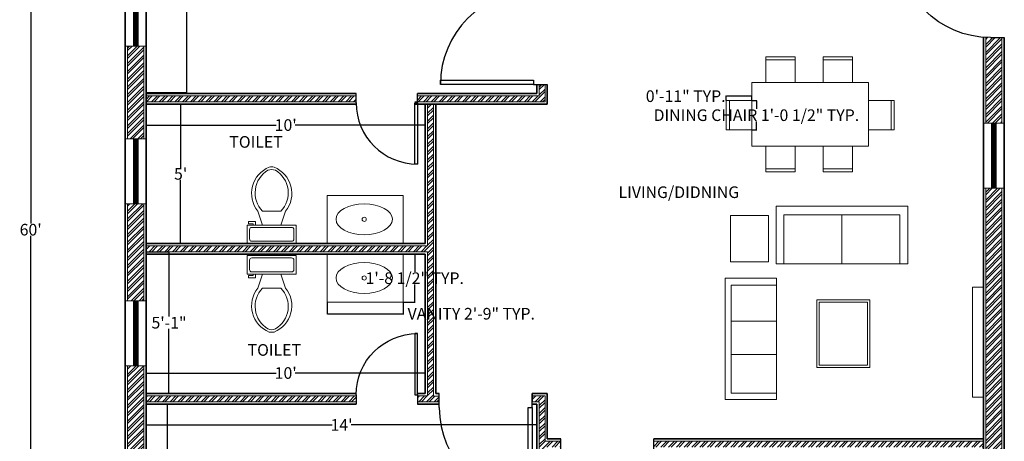
# Model space of a CAD drawing. Units: inches. Extents: x 210 to 633, y 286 to 1043.
# Tile 2 of 3: x 210 to 633, y 555 to 736. Entities that reach past the tile are written whole.
import ezdxf

# ---------------------------------------------------------------- set-up
doc = ezdxf.new("R2010")
doc.units = ezdxf.units.IN
doc.header["$MEASUREMENT"] = 0
for name, color, linetype, lineweight in [('A-ANNO-DIMS', 170, 'Continuous', 18), ('A-AREA-IDEN', 7, 'Continuous', 25), ('A-DOOR', 4, 'Continuous', 25), ('A-FLOR-FIXT', 210, 'Continuous', 18), ('A-GLAZ-PATT', 130, 'Continuous', 13), ('A-WALL-PATT', 35, 'Continuous', 13), ('fur', 210, 'Continuous', 18), ('wall', 10, 'Continuous', 35), ('wind', 130, 'Continuous', 18)]:
    doc.layers.add(name, color=color, linetype=linetype, lineweight=lineweight)
doc.styles.get("Standard").update_dxf_attribs({"font": 'arial.ttf'})
doc.dimstyles.get("Standard").update_dxf_attribs({"dimtxt": 5, "dimasz": 0.18, "dimexe": 0.18, "dimexo": 0.0625, "dimgap": 0.09, "dimtad": 0, "dimtih": 1, "dimtoh": 1, "dimdec": 0, "dimzin": 0, "dimdsep": 46, "dimlunit": 4, "dimtxsty": 'Standard', "dimcen": 0.09, "dimadec": 0, "dimazin": 0, "dimtfac": 1, "dimtdec": 0, "dimtofl": 0, "dimtmove": 0, "dimatfit": 3, "dimfxl": 1, "dimtolj": 1, "dimtzin": 0, "dimarcsym": 0})

# ---------------------------------------------------------------- blocks, each defined once
blk = doc.blocks.new('*U2')
for p, q in [((0, 0), (0, -6)), ((40, 0), (40, -6))]:
    blk.add_line(p, q)
blk.add_lwpolyline([(0, 0), (0, 40), (1.75, 40), (1.75, 0)], close=True)
blk.add_arc((0, 0), 40, 0, 90)
blk = doc.blocks.new('*U4')
for p, q in [((9.5, -6), (9.5, -2)), ((-8, -8.5), (-8, -8)), ((-7, -8), (-7, -9.5)), ((-4, -8), (-6, -14)), ((4, -8), (6, -14)), ((-10, -8.5), (-8, -8.5)), ((-10, -9.5), (-10, -8.5)), ((-7, -9.5), (-10, -9.5)), ((4, -14), (-4, -14))]:
    blk.add_line(p, q)
blk.add_lwpolyline([(10.5, -8), (10.5, 0), (-10.5, 0), (-10.5, -8)], close=True)
for points in [[(-9.5, -2), (-9.5, -6)], [(8.5, -1), (-8.5, -1)], [(-8.5, -7), (8.5, -7)]]:
    blk.add_lwpolyline(points)
for centre, radius, start, end in [((-8.62, -1.88), 0.884, 81.8699, 188.1301), ((8.62, -1.88), 0.884, 351.8699, 98.1301), ((-8.62, -6.12), 0.884, 171.8699, 278.1301), ((8.62, -6.12), 0.884, 261.8699, 8.1301), ((3.52, -21.58), 12.17, 141.4691, 247.9714), ((4.2, -21.82), 11.33, 136.3677, 238.9468), ((-3.52, -21.58), 12.17, 292.0284, 38.5307), ((-4.2, -21.82), 11.33, 301.053, 43.6321), ((0, -27.88), 4, 245.7318, 294.2682), ((0, -29), 4, 254.8605, 285.1395)]:
    blk.add_arc(centre, radius, start, end)
blk = doc.blocks.new('*D20')
at = {"layer": 'A-ANNO-DIMS', "color": 0, "lineweight": -2, "transparency": 16777216}
for p, q in [((264.44, 848.52), (282.01, 848.52)), ((281.83, 848.34), (281.83, 779.38)), ((281.83, 705.21), (281.83, 774.18)), ((264.44, 705.03), (282.01, 705.03))]:
    blk.add_line(p, q, dxfattribs=at)
at = {"layer": 'A-ANNO-DIMS', "color": 0, "transparency": 16777216}
for points in [[(281.8, 848.34), (281.86, 848.34), (281.83, 848.52)], [(281.8, 705.21), (281.86, 705.21), (281.83, 705.03)]]:
    blk.add_solid(points, dxfattribs=at)
at = {"layer": 'Defpoints', "color": 0, "transparency": 16777216}
for p in [(264.37, 848.52), (281.83, 848.52), (264.37, 705.03)]:
    blk.add_point(p, dxfattribs=at)
at = {"layer": 'A-ANNO-DIMS', "color": 0, "transparency": 16777216, "insert": (281.83, 776.78), "char_height": 5, "attachment_point": 5}
blk.add_mtext('\\A1;11\'-11"', dxfattribs=at)
blk = doc.blocks.new('*D21')
at = {"layer": 'A-ANNO-DIMS', "color": 0, "lineweight": -2, "transparency": 16777216}
for p, q in [((264.37, 699.96), (264.37, 690.83)), ((384.37, 699.96), (384.37, 690.83)), ((264.55, 691.01), (320.28, 691.01)), ((384.19, 691.01), (328.47, 691.01))]:
    blk.add_line(p, q, dxfattribs=at)
at = {"layer": 'A-ANNO-DIMS', "color": 0, "transparency": 16777216}
for points in [[(264.55, 691.04), (264.55, 690.98), (264.37, 691.01)], [(384.19, 691.04), (384.19, 690.98), (384.37, 691.01)]]:
    blk.add_solid(points, dxfattribs=at)
at = {"layer": 'Defpoints', "color": 0, "transparency": 16777216}
for p in [(264.37, 700.02), (384.37, 700.02), (384.37, 691.01)]:
    blk.add_point(p, dxfattribs=at)
at = {"layer": 'A-ANNO-DIMS', "color": 0, "transparency": 16777216, "insert": (324.37, 691.01), "char_height": 5, "attachment_point": 5}
blk.add_mtext("\\A1;10'", dxfattribs=at)
blk = doc.blocks.new('*D22')
at = {"layer": 'A-ANNO-DIMS', "color": 0, "lineweight": -2, "transparency": 16777216}
for p, q in [((264.44, 700.02), (279.37, 700.02)), ((279.19, 699.84), (279.19, 672.65)), ((279.19, 640.2), (279.19, 667.39)), ((264.44, 640.02), (279.37, 640.02))]:
    blk.add_line(p, q, dxfattribs=at)
at = {"layer": 'A-ANNO-DIMS', "color": 0, "transparency": 16777216}
for points in [[(279.16, 699.84), (279.22, 699.84), (279.19, 700.02)], [(279.16, 640.2), (279.22, 640.2), (279.19, 640.02)]]:
    blk.add_solid(points, dxfattribs=at)
at = {"layer": 'Defpoints', "color": 0, "transparency": 16777216}
for p in [(264.37, 700.02), (279.19, 700.02), (264.37, 640.02)]:
    blk.add_point(p, dxfattribs=at)
at = {"layer": 'A-ANNO-DIMS', "color": 0, "transparency": 16777216, "insert": (279.19, 670.02), "char_height": 5, "attachment_point": 5}
blk.add_mtext("\\A1;5'", dxfattribs=at)
blk = doc.blocks.new('*D23')
at = {"layer": 'A-ANNO-DIMS', "color": 0, "lineweight": -2, "transparency": 16777216}
for p, q in [((264.44, 636.52), (274.36, 636.52)), ((274.18, 636.34), (274.18, 608.66)), ((274.18, 575.7), (274.18, 603.38)), ((264.44, 575.52), (274.36, 575.52))]:
    blk.add_line(p, q, dxfattribs=at)
at = {"layer": 'A-ANNO-DIMS', "color": 0, "transparency": 16777216}
for points in [[(274.15, 636.34), (274.21, 636.34), (274.18, 636.52)], [(274.15, 575.7), (274.21, 575.7), (274.18, 575.52)]]:
    blk.add_solid(points, dxfattribs=at)
at = {"layer": 'Defpoints', "color": 0, "transparency": 16777216}
for p in [(264.37, 636.52), (274.18, 636.52), (264.37, 575.52)]:
    blk.add_point(p, dxfattribs=at)
at = {"layer": 'A-ANNO-DIMS', "color": 0, "transparency": 16777216, "insert": (274.18, 606.02), "char_height": 5, "attachment_point": 5}
blk.add_mtext('\\A1;5\'-1"', dxfattribs=at)
blk = doc.blocks.new('*D24')
at = {"layer": 'A-ANNO-DIMS', "color": 0, "lineweight": -2, "transparency": 16777216}
for p, q in [((264.37, 635.46), (264.37, 584.21)), ((384.37, 635.46), (384.37, 584.21)), ((264.55, 584.39), (320.28, 584.39)), ((384.19, 584.39), (328.47, 584.39))]:
    blk.add_line(p, q, dxfattribs=at)
at = {"layer": 'A-ANNO-DIMS', "color": 0, "transparency": 16777216}
for points in [[(264.55, 584.42), (264.55, 584.36), (264.37, 584.39)], [(384.19, 584.42), (384.19, 584.36), (384.37, 584.39)]]:
    blk.add_solid(points, dxfattribs=at)
at = {"layer": 'Defpoints', "color": 0, "transparency": 16777216}
for p in [(264.37, 635.52), (384.37, 635.52), (384.37, 584.39)]:
    blk.add_point(p, dxfattribs=at)
at = {"layer": 'A-ANNO-DIMS', "color": 0, "transparency": 16777216, "insert": (324.37, 584.39), "char_height": 5, "attachment_point": 5}
blk.add_mtext("\\A1;10'", dxfattribs=at)
blk = doc.blocks.new('*D25')
at = {"layer": 'A-ANNO-DIMS', "color": 0, "lineweight": -2, "transparency": 16777216}
for p, q in [((264.37, 570.96), (264.37, 561.9)), ((432.37, 570.96), (432.37, 561.9)), ((264.55, 562.08), (344.28, 562.08)), ((432.19, 562.08), (352.47, 562.08))]:
    blk.add_line(p, q, dxfattribs=at)
at = {"layer": 'A-ANNO-DIMS', "color": 0, "transparency": 16777216}
for points in [[(264.55, 562.11), (264.55, 562.05), (264.37, 562.08)], [(432.19, 562.11), (432.19, 562.05), (432.37, 562.08)]]:
    blk.add_solid(points, dxfattribs=at)
at = {"layer": 'Defpoints', "color": 0, "transparency": 16777216}
for p in [(264.37, 571.02), (432.37, 571.02), (432.37, 562.08)]:
    blk.add_point(p, dxfattribs=at)
at = {"layer": 'A-ANNO-DIMS', "color": 0, "transparency": 16777216, "insert": (348.37, 562.08), "char_height": 5, "attachment_point": 5}
blk.add_mtext("\\A1;14'", dxfattribs=at)
blk = doc.blocks.new('*D26')
at = {"layer": 'A-ANNO-DIMS', "color": 0, "lineweight": -2, "transparency": 16777216}
for p, q in [((264.44, 571.02), (273.63, 571.02)), ((273.45, 570.84), (273.45, 501.62)), ((273.45, 427.2), (273.45, 496.42)), ((264.44, 427.02), (273.63, 427.02))]:
    blk.add_line(p, q, dxfattribs=at)
at = {"layer": 'A-ANNO-DIMS', "color": 0, "transparency": 16777216}
for points in [[(273.42, 570.84), (273.48, 570.84), (273.45, 571.02)], [(273.42, 427.2), (273.48, 427.2), (273.45, 427.02)]]:
    blk.add_solid(points, dxfattribs=at)
at = {"layer": 'Defpoints', "color": 0, "transparency": 16777216}
for p in [(264.37, 571.02), (264.37, 427.02), (273.45, 427.02)]:
    blk.add_point(p, dxfattribs=at)
at = {"layer": 'A-ANNO-DIMS', "color": 0, "transparency": 16777216, "insert": (273.45, 499.02), "char_height": 5, "attachment_point": 5}
blk.add_mtext("\\A1;12'", dxfattribs=at)
blk = doc.blocks.new('*D36')
at = {"layer": 'A-ANNO-DIMS', "color": 0, "lineweight": -2, "transparency": 16777216}
for p, q in [((255.31, 1006.02), (214.53, 1006.02)), ((214.71, 1005.84), (214.71, 648.66)), ((214.71, 286.2), (214.71, 643.38)), ((255.31, 286.02), (214.53, 286.02))]:
    blk.add_line(p, q, dxfattribs=at)
at = {"layer": 'A-ANNO-DIMS', "color": 0, "transparency": 16777216}
for points in [[(214.68, 1005.84), (214.74, 1005.84), (214.71, 1006.02)], [(214.68, 286.2), (214.74, 286.2), (214.71, 286.02)]]:
    blk.add_solid(points, dxfattribs=at)
at = {"layer": 'Defpoints', "color": 0, "transparency": 16777216}
for p in [(214.71, 1006.02), (255.37, 1006.02), (255.37, 286.02)]:
    blk.add_point(p, dxfattribs=at)
at = {"layer": 'A-ANNO-DIMS', "color": 0, "transparency": 16777216, "insert": (214.71, 646.02), "char_height": 5, "attachment_point": 5}
blk.add_mtext("\\A1;60'", dxfattribs=at)
blk = doc.blocks.new('CHAIR-DINING')
blk.add_line((0, 9.71), (12.58, 9.71))
blk.add_lwpolyline([(0, 0), (12.58, 0), (12.58, 11.05), (0, 11.05)], close=True)
blk = doc.blocks.new('BASIN-VANITY')
blk.add_lwpolyline([(0, 0), (32.77, 0), (32.77, 20.73), (0, 20.73)], close=True)
blk.add_circle((15.97, 10.46), 0.893)
blk.add_ellipse((15.97, 10.46), major_axis=(12.12, 0), ratio=0.5487)
blk = doc.blocks.new('*D43')
at = {"layer": 'A-ANNO-DIMS', "color": 0, "lineweight": -2, "transparency": 16777216}
for p, q in [((524.94, 701.54), (526.94, 701.54)), ((526.76, 701.36), (526.76, 697.93)), ((526.76, 689.14), (526.76, 692.58)), ((524.94, 688.96), (526.94, 688.96))]:
    blk.add_line(p, q, dxfattribs=at)
at = {"layer": 'A-ANNO-DIMS', "color": 0, "transparency": 16777216}
for points in [[(526.73, 701.36), (526.79, 701.36), (526.76, 701.54)], [(526.73, 689.14), (526.79, 689.14), (526.76, 688.96)]]:
    blk.add_solid(points, dxfattribs=at)
at = {"layer": 'Defpoints', "color": 0, "transparency": 16777216}
for p in [(524.87, 701.54), (526.76, 701.54), (524.87, 688.96)]:
    blk.add_point(p, dxfattribs=at)
at = {"layer": 'A-ANNO-DIMS', "color": 0, "transparency": 16777216, "insert": (526.76, 695.25), "char_height": 5, "attachment_point": 5}
blk.add_mtext('\\A1;DINING CHAIR 1\'-0 1/2" TYP.', dxfattribs=at)
blk = doc.blocks.new('*D44')
at = {"layer": 'A-ANNO-DIMS', "color": 0, "lineweight": -2, "transparency": 16777216}
for p, q in [((513.82, 703.43), (513.64, 703.43)), ((513.82, 701.6), (513.82, 703.61)), ((524.69, 703.43), (514, 703.43)), ((524.87, 701.6), (524.87, 703.61))]:
    blk.add_line(p, q, dxfattribs=at)
at = {"layer": 'A-ANNO-DIMS', "color": 0, "transparency": 16777216}
for points in [[(514, 703.46), (514, 703.4), (513.82, 703.43)], [(524.69, 703.46), (524.69, 703.4), (524.87, 703.43)]]:
    blk.add_solid(points, dxfattribs=at)
at = {"layer": 'Defpoints', "color": 0, "transparency": 16777216}
for p in [(513.82, 703.43), (513.82, 701.54), (524.87, 701.54)]:
    blk.add_point(p, dxfattribs=at)
at = {"layer": 'A-ANNO-DIMS', "color": 0, "transparency": 16777216, "insert": (496.37, 703.43), "char_height": 5, "attachment_point": 5}
blk.add_mtext('\\A1;0\'-11" TYP.', dxfattribs=at)
blk = doc.blocks.new('*D45')
at = {"layer": 'A-ANNO-DIMS', "color": 0, "lineweight": -2, "transparency": 16777216}
for p, q in [((342.16, 614.73), (342.16, 609.7)), ((374.94, 614.73), (374.94, 609.7)), ((342.34, 609.88), (374.76, 609.88)), ((374.94, 609.88), (375.12, 609.88))]:
    blk.add_line(p, q, dxfattribs=at)
at = {"layer": 'A-ANNO-DIMS', "color": 0, "transparency": 16777216}
for points in [[(342.34, 609.91), (342.34, 609.85), (342.16, 609.88)], [(374.76, 609.91), (374.76, 609.85), (374.94, 609.88)]]:
    blk.add_solid(points, dxfattribs=at)
at = {"layer": 'Defpoints', "color": 0, "transparency": 16777216}
for p in [(342.16, 614.79), (374.94, 614.79), (374.94, 609.88)]:
    blk.add_point(p, dxfattribs=at)
at = {"layer": 'A-ANNO-DIMS', "color": 0, "transparency": 16777216, "insert": (404.16, 609.88), "char_height": 5, "attachment_point": 5}
blk.add_mtext('\\A1;VANITY 2\'-9" TYP.', dxfattribs=at)
blk = doc.blocks.new('*D46')
at = {"layer": 'A-ANNO-DIMS', "color": 0, "lineweight": -2, "transparency": 16777216}
for p, q in [((375, 635.52), (380.03, 635.52)), ((379.85, 635.34), (379.85, 627.83)), ((379.85, 614.97), (379.85, 622.48)), ((375, 614.79), (380.03, 614.79))]:
    blk.add_line(p, q, dxfattribs=at)
at = {"layer": 'A-ANNO-DIMS', "color": 0, "transparency": 16777216}
for points in [[(379.82, 635.34), (379.88, 635.34), (379.85, 635.52)], [(379.82, 614.97), (379.88, 614.97), (379.85, 614.79)]]:
    blk.add_solid(points, dxfattribs=at)
at = {"layer": 'Defpoints', "color": 0, "transparency": 16777216}
for p in [(374.94, 635.52), (379.85, 635.52), (374.94, 614.79)]:
    blk.add_point(p, dxfattribs=at)
at = {"layer": 'A-ANNO-DIMS', "color": 0, "transparency": 16777216, "insert": (379.85, 625.16), "char_height": 5, "attachment_point": 5}
blk.add_mtext('\\A1;1\'-8 1/2" TYP.', dxfattribs=at)

msp = doc.modelspace()

# ---------------------------------------------------------------- hatches: boundary and pattern name
at = {"layer": 'A-GLAZ-PATT'}
h = msp.add_hatch(dxfattribs=at)
h.set_pattern_fill('ANSI31', color=256)
h.paths.add_polyline_path([(580.59, 368.5), (495.79, 368.5), (495.79, 366.5), (580.59, 366.5)])
h.paths.add_polyline_path([(629.87, 441.57), (627.87, 441.57), (627.87, 386.08), (629.87, 386.08)])
h.paths.add_polyline_path([(260.87, 537.72), (258.87, 537.72), (258.87, 447.09), (260.87, 447.09)])
h.paths.add_polyline_path([(260.87, 615.48), (258.87, 615.48), (258.87, 587.48), (260.87, 587.48)])
h.paths.add_polyline_path([(260.87, 685.1), (258.87, 685.1), (258.87, 657.11), (260.87, 657.11)])
h.paths.add_polyline_path([(629.87, 691.84), (627.87, 691.84), (627.87, 663.85), (629.87, 663.85)])
h.paths.add_polyline_path([(260.87, 815.6), (258.87, 815.6), (258.87, 724.96), (260.87, 724.96)])
h.paths.add_polyline_path([(629.87, 831.37), (627.87, 831.37), (627.87, 803.38), (629.87, 803.38)])
h.paths.add_polyline_path([(629.87, 963.44), (627.87, 963.44), (627.87, 872.81), (629.87, 872.81)])
h.paths.add_polyline_path([(495.13, 1002.52), (448.67, 1002.52), (448.67, 1000.52), (495.13, 1000.52)])
h.paths.add_polyline_path([(417.29, 1002.52), (370.83, 1002.52), (370.83, 1000.52), (417.29, 1000.52)])
h.paths.add_polyline_path([(260.87, 971.49), (258.87, 971.49), (258.87, 880.85), (260.87, 880.85)])
at = {"layer": 'A-WALL-PATT'}
h = msp.add_hatch(dxfattribs=at)
h.set_pattern_fill('ANSI32', color=256, scale=6.3)
h.paths.add_polyline_path([(370.83, 1005.02), (256.37, 1005.02), (256.37, 971.49), (263.37, 971.49), (263.37, 998.02), (370.83, 998.02)])
h.paths.add_polyline_path([(448.67, 1005.02), (417.29, 1005.02), (417.29, 998.02), (432.37, 998.02), (448.67, 998.02)])
h.paths.add_polyline_path([(632.37, 1005.02), (495.13, 1005.02), (495.13, 998.02), (508.87, 998.02), (625.37, 998.02), (625.37, 963.44), (632.37, 963.44)])
h.paths.add_polyline_path([(263.37, 849.52), (433.37, 849.52), (433.37, 748.51), (435.87, 748.51), (435.87, 849.52), (435.87, 858.43), (433.37, 858.43), (433.37, 852.02), (263.37, 852.02), (263.37, 880.85), (256.37, 880.85), (256.37, 815.6), (263.37, 815.6)])
h.paths.add_polyline_path([(263.37, 724.96), (256.37, 724.96), (256.37, 685.1), (263.37, 685.1)])
h.paths.add_polyline_path([(354.65, 703.52), (264.37, 703.52), (264.37, 701.02), (354.65, 701.02)])
h.paths.add_polyline_path([(263.37, 657.11), (256.37, 657.11), (256.37, 615.48), (263.37, 615.48)])
h = msp.add_hatch(dxfattribs=at)
h.set_pattern_fill('ANSI32', color=256, scale=6.3)
h.paths.add_polyline_path([(551.37, 786.25), (548.87, 786.25), (548.87, 773.02), (625.37, 773.02), (625.37, 768.63), (627.37, 768.63), (632.37, 768.63), (632.37, 803.38), (625.37, 803.38), (625.37, 775.52), (551.37, 775.52)])
h.paths.add_polyline_path([(435.87, 997.02), (433.37, 997.02), (433.37, 898.43), (435.87, 898.43), (435.87, 909.52), (440.28, 909.52), (440.28, 912.02), (435.87, 912.02)])
h.paths.add_polyline_path([(512.37, 997.02), (509.87, 997.02), (509.87, 912.02), (466.62, 912.02), (466.62, 909.52), (512.37, 909.52)])
h.paths.add_polyline_path([(435.87, 708.51), (433.37, 708.51), (433.37, 703.52), (381, 703.52), (381, 701.02), (435.87, 701.02)])
h.paths.add_polyline_path([(387.87, 700.02), (385.37, 700.02), (385.37, 639.02), (264.37, 639.02), (264.37, 636.52), (385.37, 636.52), (385.37, 574.52), (381, 574.52), (381, 572.02), (390.4, 572.02), (390.4, 574.43), (387.87, 574.43), (387.87, 635.52)])
h = msp.add_hatch(dxfattribs=at)
h.set_pattern_fill('ANSI32', color=256, scale=6.3)
h.paths.add_polyline_path([(502.57, 551.52), (500.07, 551.52), (500.07, 537.88), (502.57, 537.88)])
h.paths.add_polyline_path([(632.37, 728.63), (627.37, 728.63, -0.012506), (625.37, 728.68), (625.37, 691.84), (632.37, 691.84)])
h = msp.add_hatch(dxfattribs=at)
h.set_pattern_fill('ANSI32', color=256, scale=6.3)
h.paths.add_polyline_path([(632.37, 663.85), (625.37, 663.85), (625.37, 556.02), (625.37, 441.57), (632.37, 441.57)])
h.paths.add_polyline_path([(632.37, 386.08), (625.37, 386.08), (625.37, 289.52), (625.37, 286.02), (632.37, 286.02), (632.37, 287.02)])
h.paths.add_polyline_path([(624.37, 371), (580.59, 371), (580.59, 364), (624.37, 364)])
h.paths.add_polyline_path([(495.79, 371), (436.87, 371), (436.87, 364), (495.79, 364)])
h = msp.add_hatch(dxfattribs=at)
h.set_pattern_fill('ANSI32', color=256, scale=6.3)
h.paths.add_polyline_path([(263.37, 587.48), (256.37, 587.48), (256.37, 537.72), (263.37, 537.72)])
h.paths.add_polyline_path([(354.65, 574.52), (264.37, 574.52), (264.37, 572.02), (354.65, 572.02)])
h = msp.add_hatch(dxfattribs=at)
h.set_pattern_fill('ANSI32', color=256, scale=6.3)
h.paths.add_polyline_path([(442.64, 555.02), (435.87, 555.02), (435.87, 552.52), (442.64, 552.52)])
h.paths.add_polyline_path([(435.87, 574.52), (433.37, 574.52), (433.37, 414.65), (435.87, 414.65)])
h.paths.add_polyline_path([(433.37, 574.52), (430.4, 574.52), (430.4, 572.02), (433.37, 572.02)])
h = msp.add_hatch(dxfattribs=at)
h.set_pattern_fill('ANSI32', color=256, scale=6.3)
h.paths.add_polyline_path([(624.37, 555.02), (482.64, 555.02), (482.64, 552.52), (624.37, 552.52)])

# ---------------------------------------------------------------- linework, layer by layer
for p, q in [((625.37, 728.74), (625.37, 691.84)), ((632.37, 691.84), (632.37, 728.63)), ((256.37, 724.96), (256.37, 685.1)), ((263.37, 724.96), (263.37, 685.1)), ((433.37, 703.52), (433.37, 708.51)), ((435.87, 701.02), (435.87, 708.51)), ((264.37, 703.52), (354.65, 703.52)), ((381, 703.52), (433.37, 703.52)), ((264.37, 701.02), (354.66, 701.02)), ((379.84, 701.02), (435.87, 701.02)), ((385.37, 639.02), (385.37, 700.02)), ((387.87, 635.52), (387.87, 700.02)), ((625.37, 663.85), (625.37, 556.02)), ((632.37, 441.57), (632.37, 663.85)), ((256.37, 657.11), (256.37, 615.48)), ((263.37, 657.11), (263.37, 615.48)), ((264.37, 639.02), (385.37, 639.02)), ((264.37, 636.52), (385.37, 636.52)), ((385.37, 574.52), (385.37, 636.52)), ((387.87, 574.43), (387.87, 635.52)), ((256.37, 587.48), (256.37, 537.72)), ((263.37, 587.48), (263.37, 537.72)), ((264.37, 574.52), (354.66, 574.52)), ((264.37, 572.02), (354.65, 572.02)), ((381, 574.52), (385.37, 574.52)), ((381, 572.02), (390.4, 572.02)), ((387.87, 574.43), (390.4, 574.43)), ((435.87, 574.52), (430.4, 574.52)), ((430.4, 572.02), (430.4, 574.52)), ((430.4, 574.52), (435.87, 574.52)), ((433.37, 572.02), (430.4, 572.02)), ((433.37, 572.02), (430.4, 572.02)), ((433.37, 426.02), (433.37, 572.02)), ((433.37, 426.02), (433.37, 572.02)), ((435.87, 555.02), (435.87, 574.52)), ((435.87, 574.52), (435.87, 555.02)), ((442.64, 555.02), (435.87, 555.02)), ((435.87, 555.02), (442.64, 555.02)), ((442.64, 555.02), (442.64, 552.52)), ((624.37, 555.02), (482.64, 555.02)), ((625.37, 556.02), (625.37, 441.57))]:
    msp.add_line(p, q, dxfattribs=at)
at = {"layer": 'fur'}
for p, q in [((538.5, 631.27), (538.5, 652.34)), ((538.5, 652.34), (588.43, 652.34)), ((563.47, 652.34), (563.57, 631.27)), ((588.43, 652.34), (588.43, 631.27)), ((515.96, 575.75), (515.96, 622.22)), ((515.96, 622.22), (535.48, 622.22)), ((535.48, 606.69), (515.96, 606.69)), ((535.48, 592.34), (515.96, 592.34)), ((535.48, 575.75), (515.96, 575.75))]:
    msp.add_line(p, q, dxfattribs=at)
for points in [[(575, 709.36), (524.87, 709.36), (524.87, 681.95), (575, 681.95)], [(531.93, 632.23), (515.59, 632.23), (515.59, 652.09), (531.93, 652.09)], [(535.2, 656.2), (591.94, 656.2), (591.94, 631.27), (535.2, 631.27)], [(535.48, 625.11), (513.41, 625.11), (513.41, 572.96), (535.48, 572.96)], [(624.37, 621.27), (619.7, 621.27), (619.7, 573.99), (624.37, 573.99)], [(552.78, 615.9), (575.55, 615.9), (575.55, 586.72), (552.78, 586.72)], [(553.78, 614.9), (574.55, 614.9), (574.55, 587.72), (553.78, 587.72)]]:
    msp.add_lwpolyline(points, close=True, dxfattribs=at)
at = {"layer": 'wall'}
for p, q in [((255.37, 1006.02), (255.37, 286.02)), ((264.37, 848.52), (264.37, 704.52)), ((264.37, 848.52), (264.37, 427.02)), ((624.37, 290.52), (624.37, 728.74)), ((624.37, 728.74), (624.37, 556.02)), ((624.37, 728.74), (624.37, 691.84)), ((633.37, 286.02), (633.37, 728.63)), ((633.37, 691.84), (633.37, 728.63)), ((255.37, 685.1), (255.37, 724.96)), ((264.37, 685.1), (264.37, 724.96)), ((432.37, 704.52), (432.37, 708.51)), ((432.37, 704.52), (432.37, 708.51)), ((436.87, 700.02), (436.87, 708.51)), ((436.87, 700.02), (436.87, 708.51)), ((264.37, 704.52), (354.65, 704.52)), ((264.37, 704.52), (354.65, 704.52)), ((381, 704.52), (432.37, 704.52)), ((381, 704.52), (432.37, 704.52)), ((264.37, 700.02), (354.66, 700.02)), ((264.37, 700.02), (264.37, 640.02)), ((264.37, 700.02), (354.66, 700.02)), ((379.84, 700.02), (436.87, 700.02)), ((381, 700.02), (436.87, 700.02)), ((384.37, 640.02), (384.37, 700.02)), ((384.37, 640.02), (384.37, 700.02)), ((388.87, 635.52), (388.87, 700.02)), ((388.87, 575.52), (388.87, 700.02)), ((624.37, 663.85), (624.37, 441.57)), ((633.37, 441.57), (633.37, 663.85)), ((255.37, 615.48), (255.37, 657.11)), ((264.37, 615.48), (264.37, 657.11)), ((264.37, 640.02), (384.37, 640.02)), ((264.37, 640.02), (384.37, 640.02)), ((264.37, 635.52), (384.37, 635.52)), ((264.37, 635.52), (264.37, 575.52)), ((384.37, 635.52), (264.37, 635.52)), ((384.37, 575.52), (384.37, 635.52)), ((384.37, 575.52), (384.37, 635.52)), ((388.87, 575.52), (388.87, 635.52)), ((255.37, 537.72), (255.37, 587.48)), ((264.37, 587.48), (264.37, 537.72)), ((264.37, 575.52), (354.66, 575.52)), ((354.66, 575.52), (264.37, 575.52)), ((381, 575.52), (384.37, 575.52)), ((381, 575.52), (384.37, 575.52)), ((390.4, 575.52), (388.87, 575.52)), ((390.4, 575.52), (388.87, 575.52)), ((436.87, 575.52), (430.4, 575.52)), ((436.87, 575.52), (430.4, 575.52)), ((430.4, 572.02), (430.4, 575.52)), ((436.87, 556.02), (436.87, 575.52)), ((436.87, 556.02), (436.87, 575.52)), ((264.37, 571.02), (354.65, 571.02)), ((264.37, 571.02), (264.37, 427.02)), ((264.37, 571.02), (354.65, 571.02)), ((381, 571.02), (390.4, 571.02)), ((381, 571.02), (390.4, 571.02)), ((390.4, 571.02), (388.87, 571.02)), ((432.37, 571.02), (430.4, 571.02)), ((430.4, 571.02), (432.37, 571.02)), ((432.37, 427.02), (432.37, 571.02)), ((432.37, 571.02), (432.37, 427.02)), ((442.64, 556.02), (436.87, 556.02)), ((442.64, 556.02), (436.87, 556.02)), ((624.37, 556.02), (482.64, 556.02)), ((624.37, 556.02), (482.64, 556.02))]:
    msp.add_line(p, q, dxfattribs=at)
at = {"layer": 'wind'}
for p, q in [((258.87, 724.96), (258.87, 815.6)), ((258.87, 724.96), (258.87, 815.6)), ((260.87, 724.96), (260.87, 815.6)), ((627.87, 663.85), (627.87, 691.84)), ((629.87, 663.85), (629.87, 691.84)), ((258.87, 657.11), (258.87, 685.1)), ((260.87, 657.11), (260.87, 685.1)), ((258.87, 587.48), (258.87, 615.48)), ((260.87, 587.48), (260.87, 615.48))]:
    msp.add_line(p, q, dxfattribs=at)
for points in [[(264.37, 724.96), (255.37, 724.96), (255.37, 815.6), (264.37, 815.6)], [(633.37, 691.84), (624.37, 691.84), (624.37, 663.85), (633.37, 663.85)], [(264.37, 685.1), (255.37, 685.1), (255.37, 657.11), (264.37, 657.11)], [(264.37, 615.48), (255.37, 615.48), (255.37, 587.48), (264.37, 587.48)]]:
    msp.add_lwpolyline(points, close=True, dxfattribs=at)

# ---------------------------------------------------------------- block references
at = {"layer": 'A-DOOR', "xscale": -1}
for p, rotation in [((627.37, 768.63), 90), ((442.64, 550.02), 180)]:
    msp.add_blockref('*U2', p, dxfattribs=dict(at, rotation=rotation))
at = {"layer": 'A-DOOR'}
for p, rotation in [((430.87, 708.51), 90), ((430.4, 569.52), 180)]:
    msp.add_blockref('*U2', p, dxfattribs=dict(at, rotation=rotation))
at = {"layer": 'A-DOOR', "xscale": 0.6586539344507552, "yscale": 0.6586539344507552, "zscale": 0.6586539344507552, "rotation": 180}
msp.add_blockref('*U2', (381, 700.57), dxfattribs=at)
at = {"layer": 'A-DOOR', "xscale": -0.6586539344507552, "yscale": 0.6586539344507552, "zscale": 0.6586539344507552}
msp.add_blockref('*U2', (381, 574.97), dxfattribs=at)
at = {"layer": 'A-FLOR-FIXT', "xscale": -1, "rotation": 180}
msp.add_blockref('*U4', (318.34, 640.02), dxfattribs=at)
at = {"layer": 'A-FLOR-FIXT'}
for name, p in [('BASIN-VANITY', (342.16, 640.02)), ('BASIN-VANITY', (342.16, 614.79)), ('*U4', (318.34, 634.88))]:
    msp.add_blockref(name, p, dxfattribs=at)
at = {"layer": 'fur'}
for p in [(530.8, 709.36), (555.47, 709.36)]:
    msp.add_blockref('CHAIR-DINING', p, dxfattribs=at)
at = {"layer": 'fur', "rotation": 89.9999999999991}
msp.add_blockref('CHAIR-DINING', (524.87, 688.96), dxfattribs=at)
at = {"layer": 'fur', "extrusion": (0, 0, -1), "zscale": -1}
for p, rotation in [((-575, 688.96), 89.9999999999991), ((-530.8, 681.95), 180), ((-555.47, 681.95), 180)]:
    msp.add_blockref('CHAIR-DINING', p, dxfattribs=dict(at, rotation=rotation))

# ---------------------------------------------------------------- texts
at = {"layer": 'A-AREA-IDEN', "char_height": 5, "attachment_point": 1}
for s, insert in [('TOILET', (300.13, 686.26)), ('LIVING/DIDNING', (467.5, 664.63)), ('TOILET', (307.99, 596.81))]:
    msp.add_mtext_dynamic_manual_height_columns(s, width=1430.1061, gutter_width=25, heights=[0], dxfattribs=dict(at, insert=insert))

# ---------------------------------------------------------------- dimensions: what is measured, and where the dimension line sits
at = {"layer": 'A-ANNO-DIMS'}
for base, p1, p2, picture, middle in [((214.71, 1006.02), (255.37, 286.02), (255.37, 1006.02), '*D36', (214.71, 646.02)), ((281.83, 848.52), (264.37, 705.03), (264.37, 848.52), '*D20', (281.83, 776.78)), ((279.19, 700.02), (264.37, 640.02), (264.37, 700.02), '*D22', (279.19, 670.02)), ((274.18, 636.52), (264.37, 575.52), (264.37, 636.52), '*D23', (274.18, 606.02)), ((273.45, 427.02), (264.37, 571.02), (264.37, 427.02), '*D26', (273.45, 499.02))]:
    dim = msp.add_linear_dim(base=base, p1=p1, p2=p2, angle=90, dimstyle='Standard', override={"dimclrd": 0, "dimclre": 0, "dimclrt": 0}, dxfattribs=at)
    dim.commit()
    dim.dimension.update_dxf_attribs({"geometry": picture, "text_midpoint": middle})
for base, p1, p2, angle, text, picture, middle in [((526.76, 701.54), (524.87, 688.96), (524.87, 701.54), 90, 'DINING CHAIR <> TYP.', '*D43', (526.76, 695.25)), ((513.8212, 703.4295), (524.8733, 701.5423), (513.8212, 701.5423), 180, '<> TYP.', '*D44', (496.37, 703.4295)), ((379.85, 635.52), (374.94, 614.79), (374.94, 635.52), 90, '<> TYP.', '*D46', (379.85, 625.16))]:
    dim = msp.add_linear_dim(base=base, p1=p1, p2=p2, angle=angle, text=text, dimstyle='Standard', override={"dimdec": 1, "dimlfac": 1, "dimrnd": 0, "dimzin": 1, "dimdsep": 46, "dimlunit": 4, "dimfrac": 2}, dxfattribs=at)
    dim.commit()
    dim.dimension.update_dxf_attribs({"geometry": picture, "text_midpoint": middle})
for base, p1, p2, picture, middle in [((384.37, 691.01), (264.37, 700.02), (384.37, 700.02), '*D21', (324.37, 691.01)), ((384.37, 584.39), (264.37, 635.52), (384.37, 635.52), '*D24', (324.37, 584.39)), ((432.37, 562.08), (264.37, 571.02), (432.37, 571.02), '*D25', (348.37, 562.08))]:
    dim = msp.add_linear_dim(base=base, p1=p1, p2=p2, dimstyle='Standard', override={"dimclrd": 0, "dimclre": 0, "dimclrt": 0}, dxfattribs=at)
    dim.commit()
    dim.dimension.update_dxf_attribs({"geometry": picture, "text_midpoint": middle})
dim = msp.add_linear_dim(base=(374.94, 609.88), p1=(342.16, 614.79), p2=(374.94, 614.79), text='VANITY <> TYP.', dimstyle='Standard', override={"dimdec": 1, "dimlfac": 1, "dimrnd": 0, "dimzin": 1, "dimdsep": 46, "dimlunit": 4, "dimfrac": 2}, dxfattribs=at)
dim.commit()
dim.dimension.update_dxf_attribs({"geometry": '*D45', "text_midpoint": (404.16, 609.88)})

doc.saveas('drawing.dxf')
